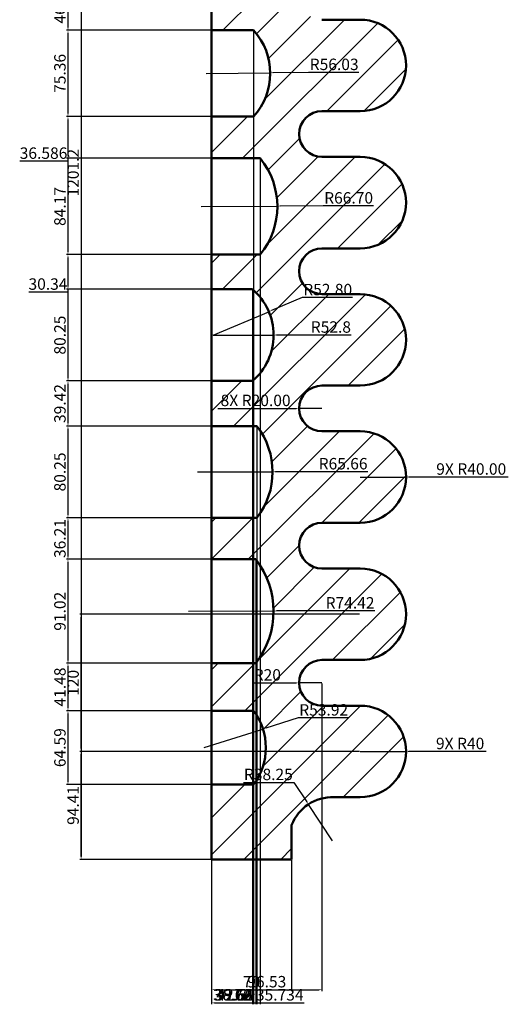
# Model space of a CAD drawing. Units: millimetres. Extents: x 1178 to 3717, y 924 to 2764.
# Tile 1 of 5: x 1178 to 1605, y 924 to 1785. Entities that reach past the tile are written whole.
import ezdxf

# ---------------------------------------------------------------- set-up
doc = ezdxf.new("R2010")
doc.units = ezdxf.units.MM
for name, color, linetype, lineweight in [('M-DIMS', 2, 'Continuous', 25), ('M-HATC', 8, 'Continuous', 18), ('M-OUTL', 7, 'Continuous', 50)]:
    doc.layers.add(name, color=color, linetype=linetype, lineweight=lineweight)
doc.styles.get("Standard").update_dxf_attribs({"font": 'arial.ttf'})
doc.dimstyles.new('ISO-25', dxfattribs={"dimtxt": 10, "dimasz": 2.5, "dimexe": 1.25, "dimexo": 0.625, "dimtad": 1, "dimtoh": 1, "dimdec": 0, "dimtxsty": 'Standard', "dimcen": 2.5, "dimadec": 0, "dimazin": 0, "dimtfac": 1, "dimtdec": 0, "dimtmove": 0, "dimatfit": 3, "dimfxl": 1, "dimarcsym": 0})

# ---------------------------------------------------------------- blocks, each defined once
blk = doc.blocks.new('*D49')
at = {"layer": 'Defpoints', "color": 0, "transparency": 16777216}
for p in [(1346.06, 2252.21), (1232.06, 1051.02), (1346.06, 1051.02)]:
    blk.add_point(p, dxfattribs=at)
at = {"layer": 'M-DIMS', "color": 0, "lineweight": -2, "transparency": 16777216}
for p, q in [((1345.44, 2252.21), (1230.81, 2252.21)), ((1232.06, 2249.71), (1232.06, 1053.52)), ((1345.44, 1051.02), (1230.81, 1051.02))]:
    blk.add_line(p, q, dxfattribs=at)
at = {"layer": 'M-DIMS', "color": 0, "transparency": 16777216}
for points in [[(1231.64, 2249.71), (1232.48, 2249.71), (1232.06, 2252.21)], [(1231.64, 1053.52), (1232.48, 1053.52), (1232.06, 1051.02)]]:
    blk.add_solid(points, dxfattribs=at)
at = {"layer": 'M-DIMS', "color": 0, "transparency": 16777216, "insert": (1226.33, 1651.62), "char_height": 10, "attachment_point": 5, "rotation": 90}
blk.add_mtext('1201.2', dxfattribs=at)
blk = doc.blocks.new('*D51')
at = {"layer": 'Defpoints', "color": 0, "transparency": 16777216}
for p in [(1346.06, 1051.02), (1416.06, 1051.02), (1416.06, 937.02)]:
    blk.add_point(p, dxfattribs=at)
at = {"layer": 'M-DIMS', "color": 0, "lineweight": -2, "transparency": 16777216}
for p, q in [((1346.06, 1050.4), (1346.06, 935.77)), ((1416.06, 1050.4), (1416.06, 935.77)), ((1348.56, 937.02), (1413.56, 937.02))]:
    blk.add_line(p, q, dxfattribs=at)
at = {"layer": 'M-DIMS', "color": 0, "transparency": 16777216}
for points in [[(1348.56, 937.44), (1348.56, 936.61), (1346.06, 937.02)], [(1413.56, 937.44), (1413.56, 936.61), (1416.06, 937.02)]]:
    blk.add_solid(points, dxfattribs=at)
at = {"layer": 'M-DIMS', "color": 0, "transparency": 16777216, "insert": (1381.06, 942.75), "char_height": 10, "attachment_point": 5}
blk.add_mtext('70', dxfattribs=at)
blk = doc.blocks.new('*D52')
at = {"layer": 'Defpoints', "color": 0, "transparency": 16777216}
for p in [(1232.06, 1145.43), (1476.06, 1145.43), (1346.06, 1051.02)]:
    blk.add_point(p, dxfattribs=at)
at = {"layer": 'M-DIMS', "color": 0, "lineweight": -2, "transparency": 16777216}
for p, q in [((1475.44, 1145.43), (1230.81, 1145.43)), ((1232.06, 1053.52), (1232.06, 1142.93)), ((1345.44, 1051.02), (1230.81, 1051.02))]:
    blk.add_line(p, q, dxfattribs=at)
at = {"layer": 'M-DIMS', "color": 0, "transparency": 16777216}
for points in [[(1231.64, 1142.93), (1232.48, 1142.93), (1232.06, 1145.43)], [(1231.64, 1053.52), (1232.48, 1053.52), (1232.06, 1051.02)]]:
    blk.add_solid(points, dxfattribs=at)
at = {"layer": 'M-DIMS', "color": 0, "transparency": 16777216, "insert": (1226.33, 1098.23), "char_height": 10, "attachment_point": 5, "rotation": 90}
blk.add_mtext('94.41', dxfattribs=at)
blk = doc.blocks.new('*D53')
at = {"layer": 'Defpoints', "color": 0, "transparency": 16777216}
for p in [(1232.06, 1265.43), (1476.07, 1265.43), (1476.06, 1145.43)]:
    blk.add_point(p, dxfattribs=at)
at = {"layer": 'M-DIMS', "color": 0, "lineweight": -2, "transparency": 16777216}
for p, q in [((1475.44, 1265.43), (1230.81, 1265.43)), ((1232.06, 1147.93), (1232.06, 1262.93)), ((1475.44, 1145.43), (1230.81, 1145.43))]:
    blk.add_line(p, q, dxfattribs=at)
at = {"layer": 'M-DIMS', "color": 0, "transparency": 16777216}
for points in [[(1231.64, 1262.93), (1232.48, 1262.93), (1232.06, 1265.43)], [(1231.64, 1147.93), (1232.48, 1147.93), (1232.06, 1145.43)]]:
    blk.add_solid(points, dxfattribs=at)
at = {"layer": 'M-DIMS', "color": 0, "transparency": 16777216, "insert": (1226.33, 1205.43), "char_height": 10, "attachment_point": 5, "rotation": 90}
blk.add_mtext('120', dxfattribs=at)
blk = doc.blocks.new('*D54')
at = {"layer": 'Defpoints', "color": 0, "transparency": 16777216}
for p in [(1346.06, 1222.53), (1442.6, 1205.43), (1442.6, 937.02)]:
    blk.add_point(p, dxfattribs=at)
at = {"layer": 'M-DIMS', "color": 0, "lineweight": -2, "transparency": 16777216}
for p, q in [((1346.06, 1221.91), (1346.06, 935.77)), ((1442.6, 1204.81), (1442.6, 935.77)), ((1348.56, 937.02), (1440.1, 937.02))]:
    blk.add_line(p, q, dxfattribs=at)
at = {"layer": 'M-DIMS', "color": 0, "transparency": 16777216}
for points in [[(1348.56, 937.44), (1348.56, 936.61), (1346.06, 937.02)], [(1440.1, 937.44), (1440.1, 936.61), (1442.6, 937.02)]]:
    blk.add_solid(points, dxfattribs=at)
at = {"layer": 'M-DIMS', "color": 0, "transparency": 16777216, "insert": (1394.33, 942.76), "char_height": 10, "attachment_point": 5}
blk.add_mtext('96.53', dxfattribs=at)
blk = doc.blocks.new('*D58')
at = {"layer": 'Defpoints', "color": 0, "transparency": 16777216}
for p in [(1476.06, 1145.43), (1516.06, 1145.4)]:
    blk.add_point(p, dxfattribs=at)
at = {"layer": 'M-DIMS', "color": 0, "lineweight": -2, "transparency": 16777216}
for p, q in [((1476.06, 1145.43), (1516.06, 1145.4)), ((1540.06, 1145.38), (1518.56, 1145.4)), ((1586.03, 1145.38), (1540.06, 1145.38))]:
    blk.add_line(p, q, dxfattribs=at)
at = {"layer": 'M-DIMS', "color": 0, "transparency": 16777216}
blk.add_solid([(1518.56, 1145.81), (1518.56, 1144.98), (1516.06, 1145.4)], dxfattribs=at)
at = {"layer": 'M-DIMS', "color": 0, "transparency": 16777216, "insert": (1563.36, 1151.11), "char_height": 10, "attachment_point": 5}
blk.add_mtext('9X R40', dxfattribs=at)
blk = doc.blocks.new('*D59')
at = {"layer": 'Defpoints', "color": 0, "transparency": 16777216}
for p in [(1422.6, 1205.4), (1442.6, 1205.43)]:
    blk.add_point(p, dxfattribs=at)
at = {"layer": 'M-DIMS', "color": 0, "lineweight": -2, "transparency": 16777216}
for p, q in [((1382.9, 1205.37), (1407.38, 1205.37)), ((1407.38, 1205.37), (1420.1, 1205.4)), ((1442.6, 1205.43), (1422.6, 1205.4))]:
    blk.add_line(p, q, dxfattribs=at)
at = {"layer": 'M-DIMS', "color": 0, "transparency": 16777216}
blk.add_solid([(1420.1, 1205.81), (1420.1, 1204.98), (1422.6, 1205.4)], dxfattribs=at)
at = {"layer": 'M-DIMS', "color": 0, "transparency": 16777216, "insert": (1394.83, 1211.1), "char_height": 10, "attachment_point": 5}
blk.add_mtext('R20', dxfattribs=at)
blk = doc.blocks.new('*D61')
at = {"layer": 'Defpoints', "color": 0, "transparency": 16777216}
for p in [(1430.67, 1099.14), (1451.73, 1067.2)]:
    blk.add_point(p, dxfattribs=at)
at = {"layer": 'M-DIMS', "color": 0, "lineweight": -2, "transparency": 16777216}
for p, q in [((1374.02, 1118.3), (1418.04, 1118.3)), ((1418.04, 1118.3), (1429.3, 1101.23)), ((1451.73, 1067.2), (1430.67, 1099.14))]:
    blk.add_line(p, q, dxfattribs=at)
at = {"layer": 'M-DIMS', "color": 0, "transparency": 16777216}
blk.add_solid([(1429.65, 1101.46), (1428.95, 1101), (1430.67, 1099.14)], dxfattribs=at)
at = {"layer": 'M-DIMS', "color": 0, "transparency": 16777216, "insert": (1395.72, 1124.04), "char_height": 10, "attachment_point": 5}
blk.add_mtext('R38.25', dxfattribs=at)
blk = doc.blocks.new('*D62')
at = {"layer": 'Defpoints', "color": 0, "transparency": 16777216}
for p in [(1347.48, 1509.56), (1400.28, 1509.6)]:
    blk.add_point(p, dxfattribs=at)
at = {"layer": 'M-DIMS', "color": 0, "lineweight": -2, "transparency": 16777216}
for p, q in [((1347.48, 1509.56), (1400.28, 1509.6)), ((1431.96, 1509.63), (1402.78, 1509.6)), ((1468.15, 1509.63), (1431.96, 1509.63))]:
    blk.add_line(p, q, dxfattribs=at)
at = {"layer": 'M-DIMS', "color": 0, "transparency": 16777216}
blk.add_solid([(1402.78, 1510.02), (1402.78, 1509.19), (1400.28, 1509.6)], dxfattribs=at)
at = {"layer": 'M-DIMS', "color": 0, "transparency": 16777216, "insert": (1450.36, 1515.36), "char_height": 10, "attachment_point": 5}
blk.add_mtext('R52.8', dxfattribs=at)
blk = doc.blocks.new('*D78')
at = {"layer": 'Defpoints', "color": 0, "transparency": 16777216}
for p in [(1346.06, 1822.13), (1220.56, 1776.13), (1346.06, 1776.13)]:
    blk.add_point(p, dxfattribs=at)
at = {"layer": 'M-DIMS', "color": 0, "lineweight": -2, "transparency": 16777216}
for p, q in [((1345.44, 1822.13), (1219.31, 1822.13)), ((1220.56, 1819.63), (1220.56, 1778.63)), ((1345.44, 1776.13), (1219.31, 1776.13))]:
    blk.add_line(p, q, dxfattribs=at)
at = {"layer": 'M-DIMS', "color": 0, "transparency": 16777216}
for points in [[(1220.14, 1819.63), (1220.98, 1819.63), (1220.56, 1822.13)], [(1220.14, 1778.63), (1220.98, 1778.63), (1220.56, 1776.13)]]:
    blk.add_solid(points, dxfattribs=at)
at = {"layer": 'M-DIMS', "color": 0, "transparency": 16777216, "insert": (1214.83, 1799.13), "char_height": 10, "attachment_point": 5, "rotation": 90}
blk.add_mtext('46.00', dxfattribs=at)
blk = doc.blocks.new('*D79')
at = {"layer": 'Defpoints', "color": 0, "transparency": 16777216}
for p in [(1346.06, 1776.13), (1220.56, 1700.78), (1346.06, 1700.78)]:
    blk.add_point(p, dxfattribs=at)
at = {"layer": 'M-DIMS', "color": 0, "lineweight": -2, "transparency": 16777216}
for p, q in [((1345.44, 1776.13), (1219.31, 1776.13)), ((1220.56, 1773.63), (1220.56, 1703.28)), ((1345.44, 1700.78), (1219.31, 1700.78))]:
    blk.add_line(p, q, dxfattribs=at)
at = {"layer": 'M-DIMS', "color": 0, "transparency": 16777216}
for points in [[(1220.14, 1773.63), (1220.98, 1773.63), (1220.56, 1776.13)], [(1220.14, 1703.28), (1220.98, 1703.28), (1220.56, 1700.78)]]:
    blk.add_solid(points, dxfattribs=at)
at = {"layer": 'M-DIMS', "color": 0, "transparency": 16777216, "insert": (1214.83, 1738.46), "char_height": 10, "attachment_point": 5, "rotation": 90}
blk.add_mtext('75.36', dxfattribs=at)
blk = doc.blocks.new('*D80')
at = {"layer": 'Defpoints', "color": 0, "transparency": 16777216}
for p in [(1346.06, 1700.78), (1220.56, 1664.19), (1346.06, 1664.19)]:
    blk.add_point(p, dxfattribs=at)
at = {"layer": 'M-DIMS', "color": 0, "lineweight": -2, "transparency": 16777216}
for p, q in [((1345.44, 1700.78), (1219.31, 1700.78)), ((1220.56, 1698.28), (1220.56, 1666.69)), ((1345.44, 1664.19), (1219.31, 1664.19)), ((1220.56, 1664.19), (1220.56, 1661.69)), ((1220.56, 1661.69), (1178.44, 1661.69))]:
    blk.add_line(p, q, dxfattribs=at)
at = {"layer": 'M-DIMS', "color": 0, "transparency": 16777216}
for points in [[(1220.14, 1698.28), (1220.98, 1698.28), (1220.56, 1700.78)], [(1220.14, 1666.69), (1220.98, 1666.69), (1220.56, 1664.19)]]:
    blk.add_solid(points, dxfattribs=at)
at = {"layer": 'M-DIMS', "color": 0, "transparency": 16777216, "insert": (1199.19, 1667.42), "char_height": 10, "attachment_point": 5}
blk.add_mtext('36.586', dxfattribs=at)
blk = doc.blocks.new('*D81')
at = {"layer": 'Defpoints', "color": 0, "transparency": 16777216}
for p in [(1346.06, 1664.19), (1220.56, 1580.02), (1346.06, 1580.02)]:
    blk.add_point(p, dxfattribs=at)
at = {"layer": 'M-DIMS', "color": 0, "lineweight": -2, "transparency": 16777216}
for p, q in [((1345.44, 1664.19), (1219.31, 1664.19)), ((1220.56, 1661.69), (1220.56, 1582.52)), ((1345.44, 1580.02), (1219.31, 1580.02))]:
    blk.add_line(p, q, dxfattribs=at)
at = {"layer": 'M-DIMS', "color": 0, "transparency": 16777216}
for points in [[(1220.14, 1661.69), (1220.98, 1661.69), (1220.56, 1664.19)], [(1220.14, 1582.52), (1220.98, 1582.52), (1220.56, 1580.02)]]:
    blk.add_solid(points, dxfattribs=at)
at = {"layer": 'M-DIMS', "color": 0, "transparency": 16777216, "insert": (1214.83, 1622.11), "char_height": 10, "attachment_point": 5, "rotation": 90}
blk.add_mtext('84.17', dxfattribs=at)
blk = doc.blocks.new('*D82')
at = {"layer": 'Defpoints', "color": 0, "transparency": 16777216}
for p in [(1346.06, 1580.02), (1220.56, 1549.68), (1346.06, 1549.68)]:
    blk.add_point(p, dxfattribs=at)
at = {"layer": 'M-DIMS', "color": 0, "lineweight": -2, "transparency": 16777216}
for p, q in [((1345.44, 1580.02), (1219.31, 1580.02)), ((1220.56, 1577.52), (1220.56, 1552.18)), ((1220.56, 1547.18), (1186.24, 1547.18)), ((1345.44, 1549.68), (1219.31, 1549.68)), ((1220.56, 1549.68), (1220.56, 1547.18))]:
    blk.add_line(p, q, dxfattribs=at)
at = {"layer": 'M-DIMS', "color": 0, "transparency": 16777216}
for points in [[(1220.14, 1577.52), (1220.98, 1577.52), (1220.56, 1580.02)], [(1220.14, 1552.18), (1220.98, 1552.18), (1220.56, 1549.68)]]:
    blk.add_solid(points, dxfattribs=at)
at = {"layer": 'M-DIMS', "color": 0, "transparency": 16777216, "insert": (1203.09, 1552.92), "char_height": 10, "attachment_point": 5}
blk.add_mtext('30.34', dxfattribs=at)
blk = doc.blocks.new('*D83')
at = {"layer": 'Defpoints', "color": 0, "transparency": 16777216}
for p in [(1346.06, 1549.68), (1220.56, 1469.43), (1346.06, 1469.43)]:
    blk.add_point(p, dxfattribs=at)
at = {"layer": 'M-DIMS', "color": 0, "lineweight": -2, "transparency": 16777216}
for p, q in [((1345.44, 1549.68), (1219.31, 1549.68)), ((1220.56, 1547.18), (1220.56, 1471.93)), ((1345.44, 1469.43), (1219.31, 1469.43))]:
    blk.add_line(p, q, dxfattribs=at)
at = {"layer": 'M-DIMS', "color": 0, "transparency": 16777216}
for points in [[(1220.14, 1547.18), (1220.98, 1547.18), (1220.56, 1549.68)], [(1220.14, 1471.93), (1220.98, 1471.93), (1220.56, 1469.43)]]:
    blk.add_solid(points, dxfattribs=at)
at = {"layer": 'M-DIMS', "color": 0, "transparency": 16777216, "insert": (1214.83, 1509.56), "char_height": 10, "attachment_point": 5, "rotation": 90}
blk.add_mtext('80.25', dxfattribs=at)
blk = doc.blocks.new('*D84')
at = {"layer": 'Defpoints', "color": 0, "transparency": 16777216}
for p in [(1346.06, 1469.43), (1220.56, 1430.01), (1346.06, 1430.01)]:
    blk.add_point(p, dxfattribs=at)
at = {"layer": 'M-DIMS', "color": 0, "lineweight": -2, "transparency": 16777216}
for p, q in [((1345.44, 1469.43), (1219.31, 1469.43)), ((1220.56, 1466.93), (1220.56, 1432.51)), ((1345.44, 1430.01), (1219.31, 1430.01))]:
    blk.add_line(p, q, dxfattribs=at)
at = {"layer": 'M-DIMS', "color": 0, "transparency": 16777216}
for points in [[(1220.14, 1466.93), (1220.98, 1466.93), (1220.56, 1469.43)], [(1220.14, 1432.51), (1220.98, 1432.51), (1220.56, 1430.01)]]:
    blk.add_solid(points, dxfattribs=at)
at = {"layer": 'M-DIMS', "color": 0, "transparency": 16777216, "insert": (1214.83, 1449.72), "char_height": 10, "attachment_point": 5, "rotation": 90}
blk.add_mtext('39.42', dxfattribs=at)
blk = doc.blocks.new('*D85')
at = {"layer": 'Defpoints', "color": 0, "transparency": 16777216}
for p in [(1346.06, 1430.01), (1220.56, 1349.76), (1346.06, 1349.76)]:
    blk.add_point(p, dxfattribs=at)
at = {"layer": 'M-DIMS', "color": 0, "lineweight": -2, "transparency": 16777216}
for p, q in [((1345.44, 1430.01), (1219.31, 1430.01)), ((1220.56, 1427.51), (1220.56, 1352.26)), ((1345.44, 1349.76), (1219.31, 1349.76))]:
    blk.add_line(p, q, dxfattribs=at)
at = {"layer": 'M-DIMS', "color": 0, "transparency": 16777216}
for points in [[(1220.14, 1427.51), (1220.98, 1427.51), (1220.56, 1430.01)], [(1220.14, 1352.26), (1220.98, 1352.26), (1220.56, 1349.76)]]:
    blk.add_solid(points, dxfattribs=at)
at = {"layer": 'M-DIMS', "color": 0, "transparency": 16777216, "insert": (1214.83, 1389.89), "char_height": 10, "attachment_point": 5, "rotation": 90}
blk.add_mtext('80.25', dxfattribs=at)
blk = doc.blocks.new('*D86')
at = {"layer": 'Defpoints', "color": 0, "transparency": 16777216}
for p in [(1346.06, 1349.76), (1220.56, 1313.55), (1346.06, 1313.55)]:
    blk.add_point(p, dxfattribs=at)
at = {"layer": 'M-DIMS', "color": 0, "lineweight": -2, "transparency": 16777216}
for p, q in [((1345.44, 1349.76), (1219.31, 1349.76)), ((1220.56, 1347.26), (1220.56, 1316.05)), ((1345.44, 1313.55), (1219.31, 1313.55))]:
    blk.add_line(p, q, dxfattribs=at)
at = {"layer": 'M-DIMS', "color": 0, "transparency": 16777216}
for points in [[(1220.14, 1347.26), (1220.98, 1347.26), (1220.56, 1349.76)], [(1220.14, 1316.05), (1220.98, 1316.05), (1220.56, 1313.55)]]:
    blk.add_solid(points, dxfattribs=at)
at = {"layer": 'M-DIMS', "color": 0, "transparency": 16777216, "insert": (1214.83, 1331.66), "char_height": 10, "attachment_point": 5, "rotation": 90}
blk.add_mtext('36.21', dxfattribs=at)
blk = doc.blocks.new('*D87')
at = {"layer": 'Defpoints', "color": 0, "transparency": 16777216}
for p in [(1346.06, 1313.55), (1220.56, 1222.53), (1346.06, 1222.53)]:
    blk.add_point(p, dxfattribs=at)
at = {"layer": 'M-DIMS', "color": 0, "lineweight": -2, "transparency": 16777216}
for p, q in [((1345.44, 1313.55), (1219.31, 1313.55)), ((1220.56, 1311.05), (1220.56, 1225.03)), ((1345.44, 1222.53), (1219.31, 1222.53))]:
    blk.add_line(p, q, dxfattribs=at)
at = {"layer": 'M-DIMS', "color": 0, "transparency": 16777216}
for points in [[(1220.14, 1311.05), (1220.98, 1311.05), (1220.56, 1313.55)], [(1220.14, 1225.03), (1220.98, 1225.03), (1220.56, 1222.53)]]:
    blk.add_solid(points, dxfattribs=at)
at = {"layer": 'M-DIMS', "color": 0, "transparency": 16777216, "insert": (1214.83, 1268.04), "char_height": 10, "attachment_point": 5, "rotation": 90}
blk.add_mtext('91.02', dxfattribs=at)
blk = doc.blocks.new('*D88')
at = {"layer": 'Defpoints', "color": 0, "transparency": 16777216}
for p in [(1346.06, 1222.53), (1220.56, 1181.05), (1346.06, 1181.05)]:
    blk.add_point(p, dxfattribs=at)
at = {"layer": 'M-DIMS', "color": 0, "lineweight": -2, "transparency": 16777216}
for p, q in [((1345.44, 1222.53), (1219.31, 1222.53)), ((1220.56, 1220.03), (1220.56, 1183.55)), ((1345.44, 1181.05), (1219.31, 1181.05))]:
    blk.add_line(p, q, dxfattribs=at)
at = {"layer": 'M-DIMS', "color": 0, "transparency": 16777216}
for points in [[(1220.14, 1220.03), (1220.98, 1220.03), (1220.56, 1222.53)], [(1220.14, 1183.55), (1220.98, 1183.55), (1220.56, 1181.05)]]:
    blk.add_solid(points, dxfattribs=at)
at = {"layer": 'M-DIMS', "color": 0, "transparency": 16777216, "insert": (1214.83, 1201.79), "char_height": 10, "attachment_point": 5, "rotation": 90}
blk.add_mtext('41.48', dxfattribs=at)
blk = doc.blocks.new('*D89')
at = {"layer": 'Defpoints', "color": 0, "transparency": 16777216}
for p in [(1346.06, 1181.05), (1220.56, 1116.46), (1346.06, 1116.46)]:
    blk.add_point(p, dxfattribs=at)
at = {"layer": 'M-DIMS', "color": 0, "lineweight": -2, "transparency": 16777216}
for p, q in [((1345.44, 1181.05), (1219.31, 1181.05)), ((1220.56, 1178.55), (1220.56, 1118.96)), ((1345.44, 1116.46), (1219.31, 1116.46))]:
    blk.add_line(p, q, dxfattribs=at)
at = {"layer": 'M-DIMS', "color": 0, "transparency": 16777216}
for points in [[(1220.14, 1178.55), (1220.98, 1178.55), (1220.56, 1181.05)], [(1220.14, 1118.96), (1220.98, 1118.96), (1220.56, 1116.46)]]:
    blk.add_solid(points, dxfattribs=at)
at = {"layer": 'M-DIMS', "color": 0, "transparency": 16777216, "insert": (1214.83, 1148.75), "char_height": 10, "attachment_point": 5, "rotation": 90}
blk.add_mtext('64.59', dxfattribs=at)
blk = doc.blocks.new('*D93')
at = {"layer": 'Defpoints', "color": 0, "transparency": 16777216}
for p in [(1346.06, 1776.13), (1382.78, 1776.13), (1382.78, 925.52)]:
    blk.add_point(p, dxfattribs=at)
at = {"layer": 'M-DIMS', "color": 0, "lineweight": -2, "transparency": 16777216}
for p, q in [((1346.06, 1775.51), (1346.06, 924.27)), ((1382.78, 1775.51), (1382.78, 924.27)), ((1348.56, 925.52), (1380.28, 925.52))]:
    blk.add_line(p, q, dxfattribs=at)
at = {"layer": 'M-DIMS', "color": 0, "transparency": 16777216}
for points in [[(1348.56, 925.94), (1348.56, 925.11), (1346.06, 925.52)], [(1380.28, 925.94), (1380.28, 925.11), (1382.78, 925.52)]]:
    blk.add_solid(points, dxfattribs=at)
at = {"layer": 'M-DIMS', "color": 0, "transparency": 16777216, "insert": (1364.42, 931.26), "char_height": 10, "attachment_point": 5}
blk.add_mtext('36.72', dxfattribs=at)
blk = doc.blocks.new('*D94')
at = {"layer": 'Defpoints', "color": 0, "transparency": 16777216}
for p in [(1346.06, 1664.19), (1388.65, 1664.19), (1388.65, 925.52)]:
    blk.add_point(p, dxfattribs=at)
at = {"layer": 'M-DIMS', "color": 0, "lineweight": -2, "transparency": 16777216}
for p, q in [((1346.06, 1663.56), (1346.06, 924.27)), ((1388.65, 1663.56), (1388.65, 924.27)), ((1348.56, 925.52), (1386.15, 925.52))]:
    blk.add_line(p, q, dxfattribs=at)
at = {"layer": 'M-DIMS', "color": 0, "transparency": 16777216}
for points in [[(1348.56, 925.94), (1348.56, 925.11), (1346.06, 925.52)], [(1386.15, 925.94), (1386.15, 925.11), (1388.65, 925.52)]]:
    blk.add_solid(points, dxfattribs=at)
at = {"layer": 'M-DIMS', "color": 0, "transparency": 16777216, "insert": (1367.36, 931.25), "char_height": 10, "attachment_point": 5}
blk.add_mtext('42.59', dxfattribs=at)
blk = doc.blocks.new('*D95')
at = {"layer": 'Defpoints', "color": 0, "transparency": 16777216}
for p in [(1346.06, 1549.68), (1381.79, 1549.68), (1381.79, 925.52)]:
    blk.add_point(p, dxfattribs=at)
at = {"layer": 'M-DIMS', "color": 0, "lineweight": -2, "transparency": 16777216}
for p, q in [((1346.06, 1549.06), (1346.06, 924.27)), ((1381.79, 1549.06), (1381.79, 924.27)), ((1348.56, 925.52), (1379.29, 925.52)), ((1381.79, 925.52), (1427.01, 925.52))]:
    blk.add_line(p, q, dxfattribs=at)
at = {"layer": 'M-DIMS', "color": 0, "transparency": 16777216}
for points in [[(1348.56, 925.94), (1348.56, 925.11), (1346.06, 925.52)], [(1379.29, 925.94), (1379.29, 925.11), (1381.79, 925.52)]]:
    blk.add_solid(points, dxfattribs=at)
at = {"layer": 'M-DIMS', "color": 0, "transparency": 16777216, "insert": (1405.65, 931.26), "char_height": 10, "attachment_point": 5}
blk.add_mtext('35.734', dxfattribs=at)
blk = doc.blocks.new('*D96')
at = {"layer": 'Defpoints', "color": 0, "transparency": 16777216}
for p in [(1346.06, 1430.01), (1385.7, 1430.01), (1385.7, 925.52)]:
    blk.add_point(p, dxfattribs=at)
at = {"layer": 'M-DIMS', "color": 0, "lineweight": -2, "transparency": 16777216}
for p, q in [((1346.06, 1429.39), (1346.06, 924.27)), ((1385.7, 1429.39), (1385.7, 924.27)), ((1348.56, 925.52), (1383.2, 925.52))]:
    blk.add_line(p, q, dxfattribs=at)
at = {"layer": 'M-DIMS', "color": 0, "transparency": 16777216}
for points in [[(1348.56, 925.94), (1348.56, 925.11), (1346.06, 925.52)], [(1383.2, 925.94), (1383.2, 925.11), (1385.7, 925.52)]]:
    blk.add_solid(points, dxfattribs=at)
at = {"layer": 'M-DIMS', "color": 0, "transparency": 16777216, "insert": (1365.88, 931.26), "char_height": 10, "attachment_point": 5}
blk.add_mtext('39.64', dxfattribs=at)
blk = doc.blocks.new('*D97')
at = {"layer": 'Defpoints', "color": 0, "transparency": 16777216}
for p in [(1346.06, 1313.55), (1384.72, 1313.55), (1384.72, 925.52)]:
    blk.add_point(p, dxfattribs=at)
at = {"layer": 'M-DIMS', "color": 0, "lineweight": -2, "transparency": 16777216}
for p, q in [((1346.06, 1312.93), (1346.06, 924.27)), ((1384.72, 1312.93), (1384.72, 924.27)), ((1348.56, 925.52), (1382.22, 925.52))]:
    blk.add_line(p, q, dxfattribs=at)
at = {"layer": 'M-DIMS', "color": 0, "transparency": 16777216}
for points in [[(1348.56, 925.94), (1348.56, 925.11), (1346.06, 925.52)], [(1382.22, 925.94), (1382.22, 925.11), (1384.72, 925.52)]]:
    blk.add_solid(points, dxfattribs=at)
at = {"layer": 'M-DIMS', "color": 0, "transparency": 16777216, "insert": (1365.39, 931.26), "char_height": 10, "attachment_point": 5}
blk.add_mtext('38.66', dxfattribs=at)
blk = doc.blocks.new('*D98')
at = {"layer": 'Defpoints', "color": 0, "transparency": 16777216}
for p in [(1346.06, 1181.05), (1382.75, 1181.05), (1382.75, 925.52)]:
    blk.add_point(p, dxfattribs=at)
at = {"layer": 'M-DIMS', "color": 0, "lineweight": -2, "transparency": 16777216}
for p, q in [((1346.06, 1180.42), (1346.06, 924.27)), ((1382.75, 1180.42), (1382.75, 924.27)), ((1348.56, 925.52), (1380.25, 925.52))]:
    blk.add_line(p, q, dxfattribs=at)
at = {"layer": 'M-DIMS', "color": 0, "transparency": 16777216}
for points in [[(1348.56, 925.94), (1348.56, 925.11), (1346.06, 925.52)], [(1380.25, 925.94), (1380.25, 925.11), (1382.75, 925.52)]]:
    blk.add_solid(points, dxfattribs=at)
at = {"layer": 'M-DIMS', "color": 0, "transparency": 16777216, "insert": (1364.41, 931.26), "char_height": 10, "attachment_point": 5}
blk.add_mtext('36.69', dxfattribs=at)
blk = doc.blocks.new('*D100')
at = {"layer": 'Defpoints', "color": 0, "transparency": 16777216}
for p in [(1476.07, 1385.43), (1516.07, 1385.43)]:
    blk.add_point(p, dxfattribs=at)
at = {"layer": 'M-DIMS', "color": 0, "lineweight": -2, "transparency": 16777216}
for p, q in [((1476.07, 1385.43), (1516.07, 1385.43)), ((1540.07, 1385.43), (1518.57, 1385.43)), ((1605.46, 1385.43), (1540.07, 1385.43))]:
    blk.add_line(p, q, dxfattribs=at)
at = {"layer": 'M-DIMS', "color": 0, "transparency": 16777216}
blk.add_solid([(1518.57, 1385.85), (1518.57, 1385.01), (1516.07, 1385.43)], dxfattribs=at)
at = {"layer": 'M-DIMS', "color": 0, "transparency": 16777216, "insert": (1573.07, 1391.16), "char_height": 10, "attachment_point": 5}
blk.add_mtext('9X R40.00', dxfattribs=at)
blk = doc.blocks.new('*D101')
at = {"layer": 'Defpoints', "color": 0, "transparency": 16777216}
for p in [(1422.6, 1445.43), (1442.6, 1445.43)]:
    blk.add_point(p, dxfattribs=at)
at = {"layer": 'M-DIMS', "color": 0, "lineweight": -2, "transparency": 16777216}
for p, q in [((1351.56, 1445.43), (1420.1, 1445.43)), ((1442.6, 1445.43), (1422.6, 1445.43))]:
    blk.add_line(p, q, dxfattribs=at)
at = {"layer": 'M-DIMS', "color": 0, "transparency": 16777216}
blk.add_solid([(1420.1, 1445.85), (1420.1, 1445.02), (1422.6, 1445.43)], dxfattribs=at)
at = {"layer": 'M-DIMS', "color": 0, "transparency": 16777216, "insert": (1384.58, 1451.16), "char_height": 10, "attachment_point": 5}
blk.add_mtext('8X R20.00', dxfattribs=at)
blk = doc.blocks.new('*D106')
at = {"layer": 'Defpoints', "color": 0, "transparency": 16777216}
for p in [(1341.31, 1738.46), (1397.34, 1739)]:
    blk.add_point(p, dxfattribs=at)
at = {"layer": 'M-DIMS', "color": 0, "lineweight": -2, "transparency": 16777216}
for p, q in [((1341.31, 1738.46), (1397.34, 1739)), ((1430.95, 1739.33), (1399.84, 1739.03)), ((1474.89, 1739.33), (1430.95, 1739.33))]:
    blk.add_line(p, q, dxfattribs=at)
at = {"layer": 'M-DIMS', "color": 0, "transparency": 16777216}
blk.add_solid([(1399.83, 1739.44), (1399.84, 1738.61), (1397.34, 1739)], dxfattribs=at)
at = {"layer": 'M-DIMS', "color": 0, "transparency": 16777216, "insert": (1453.24, 1745.06), "char_height": 10, "attachment_point": 5}
blk.add_mtext('R56.03', dxfattribs=at)
blk = doc.blocks.new('*D107')
at = {"layer": 'Defpoints', "color": 0, "transparency": 16777216}
for p in [(1336.9, 1622.11), (1403.6, 1622.4)]:
    blk.add_point(p, dxfattribs=at)
at = {"layer": 'M-DIMS', "color": 0, "lineweight": -2, "transparency": 16777216}
for p, q in [((1336.9, 1622.11), (1403.6, 1622.4)), ((1443.62, 1622.58), (1406.1, 1622.41)), ((1487.53, 1622.58), (1443.62, 1622.58))]:
    blk.add_line(p, q, dxfattribs=at)
at = {"layer": 'M-DIMS', "color": 0, "transparency": 16777216}
blk.add_solid([(1406.1, 1622.83), (1406.1, 1622), (1403.6, 1622.4)], dxfattribs=at)
at = {"layer": 'M-DIMS', "color": 0, "transparency": 16777216, "insert": (1465.89, 1628.31), "char_height": 10, "attachment_point": 5}
blk.add_mtext('R66.70', dxfattribs=at)
blk = doc.blocks.new('*D108')
at = {"layer": 'Defpoints', "color": 0, "transparency": 16777216}
for p in [(1396.13, 1530.06), (1347.48, 1509.56)]:
    blk.add_point(p, dxfattribs=at)
at = {"layer": 'M-DIMS', "color": 0, "lineweight": -2, "transparency": 16777216}
for p, q in [((1425.33, 1542.36), (1398.44, 1531.03)), ((1469.24, 1542.36), (1425.33, 1542.36)), ((1347.48, 1509.56), (1396.13, 1530.06))]:
    blk.add_line(p, q, dxfattribs=at)
at = {"layer": 'M-DIMS', "color": 0, "transparency": 16777216}
blk.add_solid([(1398.28, 1531.41), (1398.6, 1530.64), (1396.13, 1530.06)], dxfattribs=at)
at = {"layer": 'M-DIMS', "color": 0, "transparency": 16777216, "insert": (1447.6, 1548.09), "char_height": 10, "attachment_point": 5}
blk.add_mtext('R52.80', dxfattribs=at)
blk = doc.blocks.new('*D109')
at = {"layer": 'Defpoints', "color": 0, "transparency": 16777216}
for p in [(1333.73, 1389.89), (1399.39, 1390)]:
    blk.add_point(p, dxfattribs=at)
at = {"layer": 'M-DIMS', "color": 0, "lineweight": -2, "transparency": 16777216}
for p, q in [((1333.73, 1389.89), (1399.39, 1390)), ((1438.78, 1390.07), (1401.89, 1390)), ((1482.72, 1390.07), (1438.78, 1390.07))]:
    blk.add_line(p, q, dxfattribs=at)
at = {"layer": 'M-DIMS', "color": 0, "transparency": 16777216}
blk.add_solid([(1401.89, 1390.42), (1401.89, 1389.59), (1399.39, 1390)], dxfattribs=at)
at = {"layer": 'M-DIMS', "color": 0, "transparency": 16777216, "insert": (1461.06, 1395.8), "char_height": 10, "attachment_point": 5}
blk.add_mtext('R65.66', dxfattribs=at)
blk = doc.blocks.new('*D110')
at = {"layer": 'Defpoints', "color": 0, "transparency": 16777216}
for p in [(1325.84, 1268.04), (1400.26, 1268.3)]:
    blk.add_point(p, dxfattribs=at)
at = {"layer": 'M-DIMS', "color": 0, "lineweight": -2, "transparency": 16777216}
for p, q in [((1325.84, 1268.04), (1400.26, 1268.3)), ((1444.91, 1268.46), (1402.76, 1268.31)), ((1488.74, 1268.46), (1444.91, 1268.46))]:
    blk.add_line(p, q, dxfattribs=at)
at = {"layer": 'M-DIMS', "color": 0, "transparency": 16777216}
blk.add_solid([(1402.76, 1268.73), (1402.76, 1267.89), (1400.26, 1268.3)], dxfattribs=at)
at = {"layer": 'M-DIMS', "color": 0, "transparency": 16777216, "insert": (1467.14, 1274.1), "char_height": 10, "attachment_point": 5}
blk.add_mtext('R74.42', dxfattribs=at)
blk = doc.blocks.new('*D111')
at = {"layer": 'Defpoints', "color": 0, "transparency": 16777216}
for p in [(1390.99, 1165), (1339.58, 1148.75)]:
    blk.add_point(p, dxfattribs=at)
at = {"layer": 'M-DIMS', "color": 0, "lineweight": -2, "transparency": 16777216}
for p, q in [((1421.84, 1174.74), (1393.37, 1165.75)), ((1465.67, 1174.74), (1421.84, 1174.74)), ((1339.58, 1148.75), (1390.99, 1165))]:
    blk.add_line(p, q, dxfattribs=at)
at = {"layer": 'M-DIMS', "color": 0, "transparency": 16777216}
blk.add_solid([(1393.25, 1166.15), (1393.5, 1165.35), (1390.99, 1165)], dxfattribs=at)
at = {"layer": 'M-DIMS', "color": 0, "transparency": 16777216, "insert": (1444.07, 1180.48), "char_height": 10, "attachment_point": 5}
blk.add_mtext('R53.92', dxfattribs=at)

msp = doc.modelspace()

# ---------------------------------------------------------------- hatches: boundary and pattern name
at = {"layer": 'M-HATC'}
h = msp.add_hatch(dxfattribs=at)
h.set_pattern_fill('ANSI31', color=256, scale=7.2)
h.paths.add_polyline_path([(1476.0659, 2145.4337), (1442.5959, 2145.4337), (1442.5959, 2165.4337, -0.33256542), (1416.0609, 2222.2134), (1416.0609, 2252.2134), (1346.0609, 2252.2134), (1346.0609, 2126.505), (1382.7778, 2126.505, -0.35365424), (1382.7778, 2078.5493), (1346.0609, 2078.5493), (1346.0609, 1995.3607), (1381.7982, 1995.3607, -0.40006542), (1381.7982, 1945.4476), (1346.0609, 1945.4476), (1346.0609, 1896.5132), (1384.7368, 1896.5132, -0.32128688), (1384.7368, 1822.1329), (1346.0609, 1822.1329), (1346.0609, 1776.1345), (1382.7778, 1776.1345, -0.38644482), (1382.7778, 1700.7755), (1346.0609, 1700.7755), (1346.0609, 1664.1898), (1388.6514, 1664.1898, -0.35526713), (1388.6514, 1580.0226), (1346.0609, 1580.0226), (1346.0609, 1549.6833), (1381.7946, 1549.6833, -0.46058316), (1381.7946, 1469.4308), (1346.0609, 1469.4308), (1346.0609, 1430.0146), (1385.7005, 1430.0146, -0.34111668), (1385.7005, 1349.7622), (1346.0609, 1349.7622), (1346.0609, 1313.5507), (1384.7209, 1313.5507, -0.34142199), (1384.7209, 1222.5327), (1346.0609, 1222.5327), (1346.0609, 1181.0495), (1382.7495, 1181.0495, -0.3326402), (1382.7495, 1116.456), (1346.0609, 1116.456), (1346.0609, 1051.0224), (1416.0609, 1051.0224), (1416.0609, 1081.0224, -0.31910694), (1453.0456, 1105.4337), (1476.0609, 1105.4337, 1), (1476.0609, 1185.4337), (1442.5959, 1185.4337, -1), (1442.5959, 1225.4337), (1476.0659, 1225.4337, 1), (1476.0659, 1305.4337), (1442.5959, 1305.4337, -1), (1442.5959, 1345.4337), (1476.0659, 1345.4337, 1), (1476.0659, 1425.4337), (1442.5959, 1425.4337, -1), (1442.5959, 1465.4337), (1476.0659, 1465.4337, 1), (1476.0659, 1545.4337), (1442.5959, 1545.4337, -1), (1442.5959, 1585.4337), (1476.0659, 1585.4337, 1), (1476.0659, 1665.4337), (1442.5959, 1665.4337, -1), (1442.5959, 1705.4337), (1476.0659, 1705.4337, 1), (1476.0659, 1785.4337), (1442.5959, 1785.4337, -1), (1442.5959, 1825.4337), (1476.0659, 1825.4337, 1), (1476.0659, 1905.4337), (1442.5959, 1905.4337, -1), (1442.5959, 1945.4337), (1476.0659, 1945.4337, 1), (1476.0659, 2025.4337), (1442.5959, 2025.4337, -1), (1442.5959, 2065.4337), (1476.0659, 2065.4337, 1)])

# ---------------------------------------------------------------- linework, layer by layer
at = {"layer": 'M-OUTL'}
for p, q in [((1346.0609, 2252.2134), (1346.0609, 1051.0224)), ((1476.0659, 1785.4337), (1442.5959, 1785.4337)), ((1346.0609, 1776.1345), (1382.7778, 1776.1345)), ((1442.5959, 1705.4337), (1476.0659, 1705.4337)), ((1382.7778, 1700.7755), (1346.0609, 1700.7755)), ((1346.0609, 1664.1898), (1388.6514, 1664.1898)), ((1476.0659, 1665.4337), (1442.5959, 1665.4337)), ((1442.5959, 1585.4337), (1476.0659, 1585.4337)), ((1388.6514, 1580.0226), (1346.0609, 1580.0226)), ((1346.0609, 1549.6833), (1381.7946, 1549.6833)), ((1476.0659, 1545.4337), (1442.5959, 1545.4337)), ((1381.7946, 1469.4308), (1346.0609, 1469.4308)), ((1442.5959, 1465.4337), (1476.0659, 1465.4337)), ((1346.0609, 1430.0146), (1385.7005, 1430.0146)), ((1476.0659, 1425.4337), (1442.5959, 1425.4337)), ((1385.7005, 1349.7622), (1346.0609, 1349.7622)), ((1442.5959, 1345.4337), (1476.0659, 1345.4337)), ((1346.0609, 1313.5507), (1384.7209, 1313.5507)), ((1476.0659, 1305.4337), (1442.5959, 1305.4337)), ((1442.5959, 1225.4337), (1476.0659, 1225.4337)), ((1384.7209, 1222.5327), (1346.0609, 1222.5327)), ((1346.0609, 1181.0495), (1382.7495, 1181.0495)), ((1476.0609, 1185.4337), (1442.5959, 1185.4337)), ((1382.7495, 1116.456), (1346.0609, 1116.456)), ((1453.0456, 1105.4337), (1476.0609, 1105.4337)), ((1416.0609, 1051.0224), (1416.0609, 1081.0224)), ((1346.0609, 1051.0224), (1416.0609, 1051.0224))]:
    msp.add_line(p, q, dxfattribs=at)
for centre, radius, start, end in [((1476.0659, 1745.4337), 40, 270, 90), ((1341.3068, 1738.455), 56.032, 317.7424674, 42.2575326), ((1442.5959, 1685.4337), 20, 90, 270), ((1336.8988, 1622.1062), 66.7036, 320.8830929, 39.1169071), ((1476.0659, 1625.4337), 40, 270, 90), ((1442.5959, 1565.4337), 20, 90, 270), ((1347.4751, 1509.5571), 52.801, 310.5399968, 49.4600032), ((1476.0659, 1505.4337), 40, 270, 90), ((1442.5959, 1445.4337), 20, 90, 270), ((1333.7283, 1389.8884), 65.6598, 322.3292698, 37.6707302), ((1476.0659, 1385.4337), 40, 270, 90), ((1442.5959, 1325.4337), 20, 90, 270), ((1325.8435, 1268.0417), 74.4152, 322.2979342, 37.7020658), ((1476.0659, 1265.4337), 40, 270, 90), ((1442.5959, 1205.4337), 20, 90, 270), ((1339.5751, 1148.7527), 53.9176, 323.2016019, 36.7983981), ((1476.0609, 1145.4337), 40, 270, 90), ((1451.7305, 1067.2035), 38.2529, 88.029849, 158.8228241)]:
    msp.add_arc(centre, radius, start, end, dxfattribs=at)

# ---------------------------------------------------------------- dimensions: what is measured, and where the dimension line sits
at = {"layer": 'M-DIMS'}
for base, p1, p2, override, picture, middle in [((1232.0609, 1051.0224), (1346.0609, 2252.2134), (1346.0609, 1051.0224), {"dimdec": 1, "dimlfac": 1, "dimrnd": 0, "dimzin": 0, "dimdsep": 46, "dimlunit": 2}, '*D49', (1226.3302, 1651.6179)), ((1220.5609, 1776.1345), (1346.0609, 1822.1329), (1346.0609, 1776.1345), {"dimdec": 2, "dimlfac": 1, "dimrnd": 0, "dimzin": 0, "dimdsep": 46, "dimlunit": 2}, '*D78', (1214.8302, 1799.1337)), ((1220.5609, 1700.7755), (1346.0609, 1776.1345), (1346.0609, 1700.7755), {"dimdec": 2, "dimlfac": 1, "dimrnd": 0, "dimzin": 0, "dimdsep": 46, "dimlunit": 2}, '*D79', (1214.8268, 1738.455)), ((1220.5609, 1664.1898), (1346.0609, 1700.7755), (1346.0609, 1664.1898), {"dimdec": 3, "dimlfac": 1, "dimrnd": 0, "dimzin": 0, "dimdsep": 46, "dimlunit": 2}, '*D80', (1199.1856, 1667.424)), ((1220.5609, 1580.0226), (1346.0609, 1664.1898), (1346.0609, 1580.0226), {"dimdec": 2, "dimlfac": 1, "dimrnd": 0, "dimzin": 0, "dimdsep": 46, "dimlunit": 2}, '*D81', (1214.8302, 1622.1062)), ((1220.5609, 1549.6833), (1346.0609, 1580.0226), (1346.0609, 1549.6833), {"dimdec": 2, "dimlfac": 1, "dimrnd": 0, "dimzin": 0, "dimdsep": 46, "dimlunit": 2}, '*D82', (1203.0873, 1552.9174)), ((1220.5609, 1469.4308), (1346.0609, 1549.6833), (1346.0609, 1469.4308), {"dimdec": 2, "dimlfac": 1, "dimrnd": 0, "dimzin": 0, "dimdsep": 46, "dimlunit": 2}, '*D83', (1214.8302, 1509.5571)), ((1220.5609, 1430.0146), (1346.0609, 1469.4308), (1346.0609, 1430.0146), {"dimdec": 2, "dimlfac": 1, "dimrnd": 0, "dimzin": 0, "dimdsep": 46, "dimlunit": 2}, '*D84', (1214.8268, 1449.7227)), ((1220.5609, 1349.7622), (1346.0609, 1430.0146), (1346.0609, 1349.7622), {"dimdec": 2, "dimlfac": 1, "dimrnd": 0, "dimzin": 0, "dimdsep": 46, "dimlunit": 2}, '*D85', (1214.8302, 1389.8884)), ((1220.5609, 1313.5507), (1346.0609, 1349.7622), (1346.0609, 1313.5507), {"dimdec": 2, "dimlfac": 1, "dimrnd": 0, "dimzin": 0, "dimdsep": 46, "dimlunit": 2}, '*D86', (1214.8268, 1331.6564)), ((1220.5609, 1222.5327), (1346.0609, 1313.5507), (1346.0609, 1222.5327), {"dimdec": 2, "dimlfac": 1, "dimrnd": 0, "dimzin": 0, "dimdsep": 46, "dimlunit": 2}, '*D87', (1214.8302, 1268.0417)), ((1232.0609, 1265.4337), (1476.0609, 1145.4337), (1476.0659, 1265.4337), {"dimdec": 0, "dimlfac": 1, "dimrnd": 0, "dimzin": 0, "dimdsep": 46, "dimlunit": 2}, '*D53', (1226.3302, 1205.4337)), ((1220.5609, 1181.0495), (1346.0609, 1222.5327), (1346.0609, 1181.0495), {"dimdec": 2, "dimlfac": 1, "dimrnd": 0, "dimzin": 0, "dimdsep": 46, "dimlunit": 2}, '*D88', (1214.8302, 1201.7911)), ((1220.5609, 1116.456), (1346.0609, 1181.0495), (1346.0609, 1116.456), {"dimdec": 2, "dimlfac": 1, "dimrnd": 0, "dimzin": 0, "dimdsep": 46, "dimlunit": 2}, '*D89', (1214.8302, 1148.7527)), ((1232.0609, 1145.4337), (1346.0609, 1051.0224), (1476.0609, 1145.4337), {"dimdec": 2, "dimlfac": 1, "dimrnd": 0, "dimzin": 0, "dimdsep": 46, "dimlunit": 2}, '*D52', (1226.3302, 1098.2281))]:
    dim = msp.add_linear_dim(base=base, p1=p1, p2=p2, angle=90, dimstyle='ISO-25', override=override, dxfattribs=at)
    dim.commit()
    dim.dimension.update_dxf_attribs({"geometry": picture, "text_midpoint": middle})
for base, p1, p2, override, picture, middle in [((1382.7778, 925.5224), (1346.0609, 1776.1345), (1382.7778, 1776.1345), {"dimdec": 2, "dimlfac": 1, "dimrnd": 0, "dimzin": 0, "dimdsep": 46, "dimlunit": 2}, '*D93', (1364.4193, 931.2566)), ((1388.6514, 925.5224), (1346.0609, 1664.1898), (1388.6514, 1664.1898), {"dimdec": 2, "dimlfac": 1, "dimrnd": 0, "dimzin": 0, "dimdsep": 46, "dimlunit": 2}, '*D94', (1367.3562, 931.2532)), ((1381.7946, 925.5224), (1346.0609, 1549.6833), (1381.7946, 1549.6833), {"dimdec": 3, "dimlfac": 1, "dimrnd": 0, "dimzin": 0, "dimdsep": 46, "dimlunit": 2}, '*D95', (1405.6529, 931.2566)), ((1385.7005, 925.5224), (1346.0609, 1430.0146), (1385.7005, 1430.0146), {"dimdec": 2, "dimlfac": 1, "dimrnd": 0, "dimzin": 0, "dimdsep": 46, "dimlunit": 2}, '*D96', (1365.8807, 931.2566)), ((1384.7209, 925.5224), (1346.0609, 1313.5507), (1384.7209, 1313.5507), {"dimdec": 2, "dimlfac": 1, "dimrnd": 0, "dimzin": 0, "dimdsep": 46, "dimlunit": 2}, '*D97', (1365.3909, 931.2566)), ((1442.59586, 937.02243), (1346.06091, 1222.53269), (1442.59586, 1205.43372), {"dimdec": 2, "dimlfac": 1, "dimrnd": 0, "dimzin": 0, "dimdsep": 46, "dimlunit": 2}, '*D54', (1394.32839, 942.75657)), ((1382.7495, 925.5224), (1346.0609, 1181.0495), (1382.7495, 1181.0495), {"dimdec": 2, "dimlfac": 1, "dimrnd": 0, "dimzin": 0, "dimdsep": 46, "dimlunit": 2}, '*D98', (1364.4052, 931.2566)), ((1416.0609, 937.0224), (1346.0609, 1051.0224), (1416.0609, 1051.0224), {"dimdec": 0, "dimlfac": 1, "dimrnd": 0, "dimzin": 0, "dimdsep": 46, "dimlunit": 2}, '*D51', (1381.0609, 942.7532))]:
    dim = msp.add_linear_dim(base=base, p1=p1, p2=p2, dimstyle='ISO-25', override=override, dxfattribs=at)
    dim.commit()
    dim.dimension.update_dxf_attribs({"geometry": picture, "text_midpoint": middle})
for center, mpoint, override, picture, middle in [((1341.3068, 1738.455), (1397.3361, 1739.0023), {"dimdec": 2, "dimlfac": 1, "dimrnd": 0, "dimzin": 0, "dimdsep": 46, "dimlunit": 2}, '*D106', (1430.9537, 1739.3307)), ((1336.8988, 1622.1062), (1403.6017, 1622.4009), {"dimdec": 2, "dimlfac": 1, "dimrnd": 0, "dimzin": 0, "dimdsep": 46, "dimlunit": 2}, '*D107', (1443.6235, 1622.5777)), ((1347.4751, 1509.5571), (1396.1343, 1530.0566), {"dimdec": 2, "dimlfac": 1, "dimrnd": 0, "dimzin": 0, "dimdsep": 46, "dimlunit": 2}, '*D108', (1447.5953, 1542.3563)), ((1347.4751, 1509.5571), (1400.2761, 1509.6), {"dimdec": 1, "dimlfac": 1, "dimrnd": 0, "dimzin": 0, "dimdsep": 46, "dimlunit": 2}, '*D62', (1431.9566, 1509.6257)), ((1333.7283, 1389.8884), (1399.3881, 1390.0002), {"dimdec": 2, "dimlfac": 1, "dimrnd": 0, "dimzin": 0, "dimdsep": 46, "dimlunit": 2}, '*D109', (1438.784, 1390.0672)), ((1325.8435, 1268.0417), (1400.2583, 1268.3009), {"dimdec": 2, "dimlfac": 1, "dimrnd": 0, "dimzin": 0, "dimdsep": 46, "dimlunit": 2}, '*D110', (1444.9071, 1268.4564)), ((1339.5751, 1148.7527), (1390.9877, 1164.9961), {"dimdec": 2, "dimlfac": 1, "dimrnd": 0, "dimzin": 0, "dimdsep": 46, "dimlunit": 2}, '*D111', (1444.0668, 1174.7422)), ((1451.7305, 1067.2035), (1430.674, 1099.1394), {"dimdec": 2, "dimlfac": 1, "dimrnd": 0, "dimzin": 0, "dimdsep": 46, "dimlunit": 2}, '*D61', (1395.72, 1118.301))]:
    dim = msp.add_radius_dim(center=center, mpoint=mpoint, dimstyle='ISO-25', override=override, dxfattribs=at)
    dim.commit()
    dim.dimension.update_dxf_attribs({"geometry": picture, "text_midpoint": middle, "dimtype": 164})
dim = msp.add_radius_dim(center=(1442.5959, 1445.4337), mpoint=(1422.5959, 1445.4337), text='8X <>', dimstyle='ISO-25', override={"dimdec": 2, "dimlfac": 1, "dimrnd": 0, "dimzin": 0, "dimdsep": 46, "dimlunit": 2}, dxfattribs=at)
dim.commit()
dim.dimension.update_dxf_attribs({"geometry": '*D101', "text_midpoint": (1384.58, 1451.1645)})
for center, mpoint, override, picture, middle in [((1476.0659, 1385.4337), (1516.0659, 1385.43), {"dimdec": 2, "dimlfac": 1, "dimrnd": 0, "dimzin": 0, "dimdsep": 46, "dimlunit": 2}, '*D100', (1540.0659, 1385.4278)), ((1476.0609, 1145.4337), (1516.0609, 1145.3999), {"dimdec": 0, "dimlfac": 1, "dimrnd": 0, "dimzin": 0, "dimdsep": 46, "dimlunit": 2}, '*D58', (1540.0609, 1145.3797))]:
    dim = msp.add_radius_dim(center=center, mpoint=mpoint, text='9X <>', dimstyle='ISO-25', override=override, dxfattribs=at)
    dim.commit()
    dim.dimension.update_dxf_attribs({"geometry": picture, "text_midpoint": middle, "dimtype": 164})
dim = msp.add_radius_dim(center=(1442.5959, 1205.4337), mpoint=(1422.5959, 1205.3993), dimstyle='ISO-25', override={"dimdec": 0, "dimlfac": 1, "dimrnd": 0, "dimzin": 0, "dimdsep": 46, "dimlunit": 2}, dxfattribs=at)
dim.commit()
dim.dimension.update_dxf_attribs({"geometry": '*D59', "text_midpoint": (1394.829, 1211.1039)})

doc.saveas('drawing.dxf')
